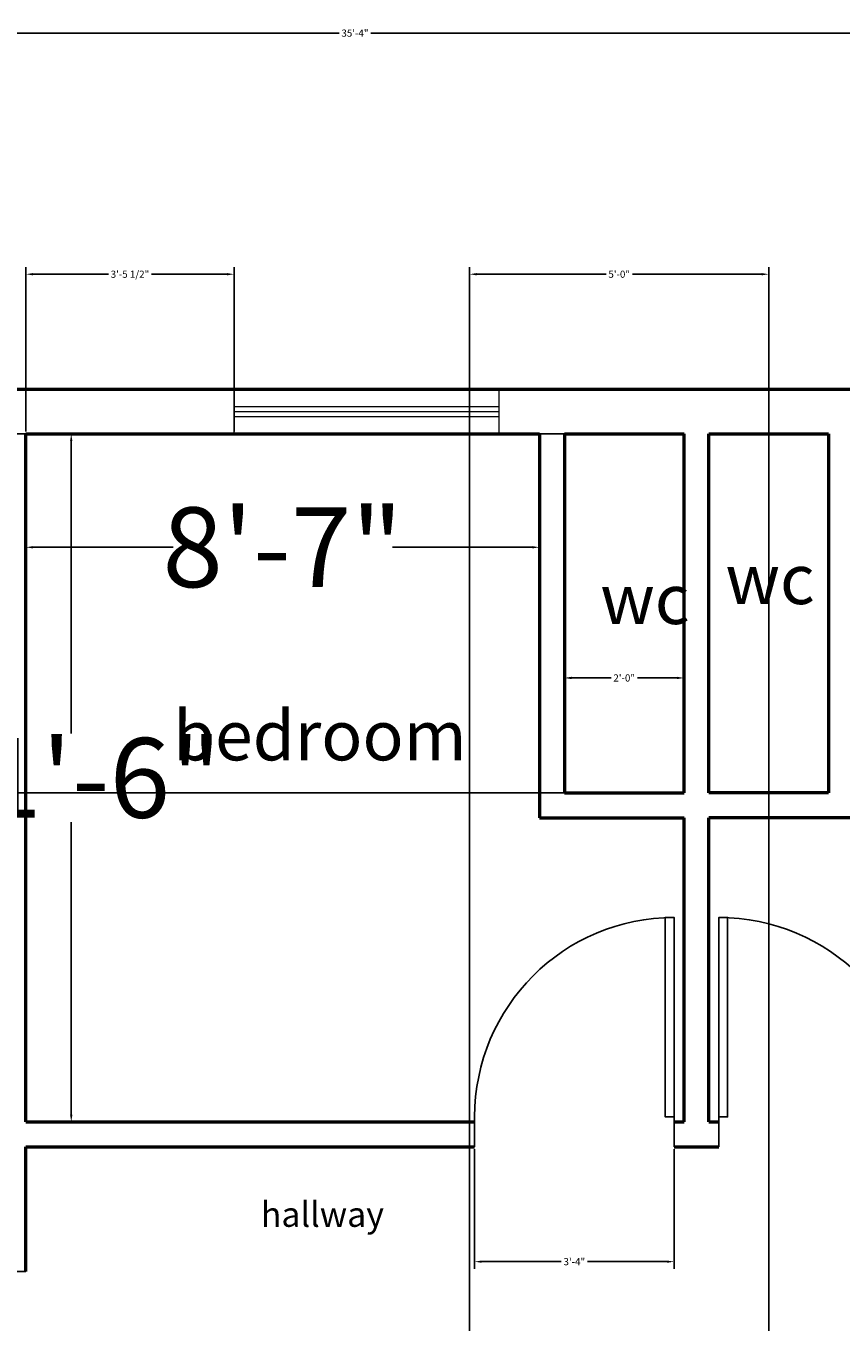
# Model space of a CAD drawing. Units: inches. Extents: x 325 to 804, y 366 to 834.
# Tile 5 of 6: x 496 to 660, y 574 to 834. Entities that reach past the tile are written whole.
import ezdxf

# ---------------------------------------------------------------- set-up
doc = ezdxf.new("R2010")
doc.units = ezdxf.units.IN
doc.header["$MEASUREMENT"] = 0
doc.layers.get('0').update_dxf_attribs({"color": 4})
for name, color, linetype, lineweight in [('A-ANNO-DIMS', 2, 'Continuous', 18), ('A-AREA-IDEN', 7, 'Continuous', 25), ('A-WALL', 7, 'Continuous', 50), ('door', 10, 'Continuous', 25), ('window', 3, 'Continuous', 18)]:
    doc.layers.add(name, color=color, linetype=linetype, lineweight=lineweight)
doc.styles.get("Standard").update_dxf_attribs({"font": 'arial.ttf'})
doc.dimstyles.get("Standard").update_dxf_attribs({"dimscale": 8, "dimtxt": 0.18, "dimasz": 0.18, "dimexe": 0.18, "dimexo": 0.0625, "dimgap": 0.09, "dimtad": 0, "dimtih": 1, "dimtoh": 1, "dimdec": 0, "dimzin": 0, "dimdsep": 46, "dimlunit": 3, "dimtxsty": 'Standard', "dimcen": 0.09, "dimadec": 0, "dimazin": 0, "dimtfac": 1, "dimtdec": 0, "dimtofl": 0, "dimtmove": 0, "dimatfit": 3, "dimfxl": 1, "dimtolj": 1, "dimtzin": 0, "dimarcsym": 0})

# ---------------------------------------------------------------- blocks, each defined once
blk = doc.blocks.new('*U2')
for p, q in [((0, 0), (0, -6)), ((-40, 0), (-40, -6))]:
    blk.add_line(p, q)
blk.add_lwpolyline([(0, 0), (0, 40), (-1.75, 40), (-1.75, 0)], close=True)
blk.add_arc((0, 0), 40, 90, 180)
blk = doc.blocks.new('*U3')
for p, q in [((0, 0), (0, -6)), ((40, 0), (40, -6))]:
    blk.add_line(p, q)
blk.add_lwpolyline([(0, 0), (0, 40), (1.75, 40), (1.75, 0)], close=True)
blk.add_arc((0, 0), 40, 0, 90)
blk = doc.blocks.new('*D11')
at = {"layer": 'A-ANNO-DIMS', "color": 0, "lineweight": -2, "transparency": 16777216}
for p, q in [((496.47, 752.04), (496.47, 728.37)), ((599.47, 752.04), (599.47, 728.37)), ((497.91, 729.81), (525.98, 729.81)), ((598.03, 729.81), (569.97, 729.81))]:
    blk.add_line(p, q, dxfattribs=at)
at = {"layer": 'A-ANNO-DIMS', "color": 0, "transparency": 16777216}
for points in [[(497.91, 730.05), (497.91, 729.57), (496.47, 729.81)], [(598.03, 730.05), (598.03, 729.57), (599.47, 729.81)]]:
    blk.add_solid(points, dxfattribs=at)
at = {"layer": 'Defpoints', "color": 0, "transparency": 16777216}
for p in [(496.47, 752.54), (599.47, 752.54), (599.47, 729.81)]:
    blk.add_point(p, dxfattribs=at)
at = {"layer": 'A-ANNO-DIMS', "color": 0, "transparency": 16777216, "insert": (547.97, 729.81), "char_height": 1.44, "attachment_point": 5}
blk.add_mtext('\\A1;{\\H11.11111x;8\'-7"}', dxfattribs=at)
blk = doc.blocks.new('*D12')
at = {"layer": 'A-ANNO-DIMS', "color": 0, "lineweight": -2, "transparency": 16777216}
for p, q in [((496.97, 752.54), (507, 752.54)), ((505.56, 751.1), (505.56, 692.43)), ((505.56, 615.98), (505.56, 674.65)), ((496.97, 614.54), (507, 614.54))]:
    blk.add_line(p, q, dxfattribs=at)
at = {"layer": 'A-ANNO-DIMS', "color": 0, "transparency": 16777216}
for points in [[(505.32, 751.1), (505.8, 751.1), (505.56, 752.54)], [(505.32, 615.98), (505.8, 615.98), (505.56, 614.54)]]:
    blk.add_solid(points, dxfattribs=at)
at = {"layer": 'Defpoints', "color": 0, "transparency": 16777216}
for p in [(496.47, 752.54), (505.56, 752.54), (496.47, 614.54)]:
    blk.add_point(p, dxfattribs=at)
at = {"layer": 'A-ANNO-DIMS', "color": 0, "transparency": 16777216, "insert": (505.56, 683.54), "char_height": 1.44, "attachment_point": 5}
blk.add_mtext('\\A1;{\\H11.11111x;11\'-6"}', dxfattribs=at)
blk = doc.blocks.new('*D25')
at = {"layer": 'A-ANNO-DIMS', "color": 0, "lineweight": -2, "transparency": 16777216}
for p, q in [((350.47, 762.04), (350.47, 834.4)), ((351.91, 832.96), (559.28, 832.96)), ((773.03, 832.96), (565.67, 832.96)), ((774.47, 762.04), (774.47, 834.4))]:
    blk.add_line(p, q, dxfattribs=at)
at = {"layer": 'A-ANNO-DIMS', "color": 0, "transparency": 16777216}
for points in [[(351.91, 833.2), (351.91, 832.72), (350.47, 832.96)], [(773.03, 833.2), (773.03, 832.72), (774.47, 832.96)]]:
    blk.add_solid(points, dxfattribs=at)
at = {"layer": 'Defpoints', "color": 0, "transparency": 16777216}
for p in [(774.47, 832.96), (350.47, 761.54), (774.47, 761.54)]:
    blk.add_point(p, dxfattribs=at)
at = {"layer": 'A-ANNO-DIMS', "color": 0, "transparency": 16777216, "insert": (562.47, 832.96), "char_height": 1.44, "attachment_point": 5}
blk.add_mtext('\\A1;35\'-4"', dxfattribs=at)
blk = doc.blocks.new('WIN-53_14x9')
for p, q in [((0, 5.5), (53.14, 5.5)), ((0, 4.5), (53.14, 4.5)), ((0, 3.5), (53.14, 3.5))]:
    blk.add_line(p, q)
blk.add_lwpolyline([(0, 9), (53.14, 9), (53.14, 0), (0, 0)], close=True)
blk = doc.blocks.new('*D31')
at = {"layer": 'A-ANNO-DIMS', "color": 0, "lineweight": -2, "transparency": 16777216}
for p, q in [((496.47, 753.04), (496.47, 786.03)), ((538.21, 753.04), (538.21, 786.03)), ((497.91, 784.59), (513.03, 784.59)), ((536.77, 784.59), (521.65, 784.59))]:
    blk.add_line(p, q, dxfattribs=at)
at = {"layer": 'A-ANNO-DIMS', "color": 0, "transparency": 16777216}
for points in [[(497.91, 784.83), (497.91, 784.35), (496.47, 784.59)], [(536.77, 784.83), (536.77, 784.35), (538.21, 784.59)]]:
    blk.add_solid(points, dxfattribs=at)
at = {"layer": 'Defpoints', "color": 0, "transparency": 16777216}
for p in [(538.21, 784.59), (496.47, 752.54), (538.21, 752.54)]:
    blk.add_point(p, dxfattribs=at)
at = {"layer": 'A-ANNO-DIMS', "color": 0, "transparency": 16777216, "insert": (517.34, 784.59), "char_height": 1.44, "attachment_point": 5}
blk.add_mtext('\\A1;3\'-5 1/2"', dxfattribs=at)
blk = doc.blocks.new('*D36')
at = {"layer": 'A-ANNO-DIMS', "color": 0, "lineweight": -2, "transparency": 16777216}
for p, q in [((604.47, 681.04), (604.47, 705.03)), ((628.47, 681.04), (628.47, 705.03)), ((605.91, 703.59), (613.83, 703.59)), ((627.03, 703.59), (619.12, 703.59))]:
    blk.add_line(p, q, dxfattribs=at)
at = {"layer": 'A-ANNO-DIMS', "color": 0, "transparency": 16777216}
for points in [[(605.91, 703.83), (605.91, 703.35), (604.47, 703.59)], [(627.03, 703.83), (627.03, 703.35), (628.47, 703.59)]]:
    blk.add_solid(points, dxfattribs=at)
at = {"layer": 'Defpoints', "color": 0, "transparency": 16777216}
for p in [(628.47, 703.59), (604.47, 680.54), (628.47, 680.54)]:
    blk.add_point(p, dxfattribs=at)
at = {"layer": 'A-ANNO-DIMS', "color": 0, "transparency": 16777216, "insert": (616.47, 703.59), "char_height": 1.44, "attachment_point": 5}
blk.add_mtext('\\A1;2\'-0"', dxfattribs=at)
blk = doc.blocks.new('*D37')
at = {"layer": 'A-ANNO-DIMS', "color": 0, "lineweight": -2, "transparency": 16777216}
for p, q in [((627.97, 752.54), (325.98, 752.54)), ((327.42, 751.1), (327.42, 717.99)), ((327.42, 681.98), (327.42, 715.08)), ((627.97, 680.54), (325.98, 680.54))]:
    blk.add_line(p, q, dxfattribs=at)
at = {"layer": 'A-ANNO-DIMS', "color": 0, "transparency": 16777216}
for points in [[(327.18, 751.1), (327.66, 751.1), (327.42, 752.54)], [(327.18, 681.98), (327.66, 681.98), (327.42, 680.54)]]:
    blk.add_solid(points, dxfattribs=at)
at = {"layer": 'Defpoints', "color": 0, "transparency": 16777216}
for p in [(327.42, 752.54), (628.47, 752.54), (628.47, 680.54)]:
    blk.add_point(p, dxfattribs=at)
at = {"layer": 'A-ANNO-DIMS', "color": 0, "transparency": 16777216, "insert": (327.42, 716.54), "char_height": 1.44, "attachment_point": 5}
blk.add_mtext('\\A1;6\'-0"', dxfattribs=at)
blk = doc.blocks.new('*D38')
at = {"layer": 'A-ANNO-DIMS', "color": 0, "lineweight": -2, "transparency": 16777216}
for p, q in [((585.47, 401.04), (585.47, 786.03)), ((645.47, 401.04), (645.47, 786.03)), ((586.91, 784.59), (612.84, 784.59)), ((644.03, 784.59), (618.11, 784.59))]:
    blk.add_line(p, q, dxfattribs=at)
at = {"layer": 'A-ANNO-DIMS', "color": 0, "transparency": 16777216}
for points in [[(586.91, 784.83), (586.91, 784.35), (585.47, 784.59)], [(644.03, 784.83), (644.03, 784.35), (645.47, 784.59)]]:
    blk.add_solid(points, dxfattribs=at)
at = {"layer": 'Defpoints', "color": 0, "transparency": 16777216}
for p in [(645.47, 784.59), (585.47, 400.54), (645.47, 400.54)]:
    blk.add_point(p, dxfattribs=at)
at = {"layer": 'A-ANNO-DIMS', "color": 0, "transparency": 16777216, "insert": (615.47, 784.59), "char_height": 1.44, "attachment_point": 5}
blk.add_mtext('\\A1;5\'-0"', dxfattribs=at)
blk = doc.blocks.new('*D40')
at = {"layer": 'A-ANNO-DIMS', "color": 0, "lineweight": -2, "transparency": 16777216}
for p, q in [((586.47, 609.04), (586.47, 585.05)), ((626.47, 609.04), (626.47, 585.05)), ((587.91, 586.49), (603.84, 586.49)), ((625.03, 586.49), (609.11, 586.49))]:
    blk.add_line(p, q, dxfattribs=at)
at = {"layer": 'A-ANNO-DIMS', "color": 0, "transparency": 16777216}
for points in [[(587.91, 586.73), (587.91, 586.25), (586.47, 586.49)], [(625.03, 586.73), (625.03, 586.25), (626.47, 586.49)]]:
    blk.add_solid(points, dxfattribs=at)
at = {"layer": 'Defpoints', "color": 0, "transparency": 16777216}
for p in [(586.47, 609.54), (626.47, 609.54), (586.47, 586.49)]:
    blk.add_point(p, dxfattribs=at)
at = {"layer": 'A-ANNO-DIMS', "color": 0, "transparency": 16777216, "insert": (606.47, 586.49), "char_height": 1.44, "attachment_point": 5}
blk.add_mtext('\\A1;3\'-4"', dxfattribs=at)

msp = doc.modelspace()

# ---------------------------------------------------------------- linework, layer by layer
at = {"layer": 'A-WALL'}
for p, q in [((350.47, 761.54), (774.47, 761.54)), ((496.47, 752.54), (599.47, 752.54)), ((496.47, 614.54), (496.47, 752.54)), ((599.47, 752.54), (599.47, 675.54)), ((604.47, 752.54), (604.47, 680.54)), ((604.47, 752.54), (628.47, 752.54)), ((628.47, 680.54), (628.47, 752.54)), ((633.47, 752.54), (657.47, 752.54)), ((633.47, 680.54), (633.47, 752.54)), ((657.47, 752.54), (657.47, 680.54)), ((604.47, 680.54), (628.47, 680.54)), ((657.47, 680.54), (633.47, 680.54)), ((599.47, 675.54), (628.47, 675.54)), ((628.47, 614.54), (628.47, 675.54)), ((633.47, 614.54), (633.47, 675.54)), ((662.47, 675.54), (633.47, 675.54)), ((496.47, 614.54), (586.47, 614.54)), ((626.47, 614.54), (628.47, 614.54)), ((633.47, 614.54), (635.47, 614.54)), ((496.47, 609.54), (586.47, 609.54)), ((496.47, 584.54), (496.47, 609.54)), ((626.47, 609.54), (635.47, 609.54))]:
    msp.add_line(p, q, dxfattribs=at)
at = {"layer": 'door'}
for p, q in [((626.47, 614.54), (626.47, 609.54)), ((635.47, 614.54), (635.47, 609.54))]:
    msp.add_line(p, q, dxfattribs=at)

# ---------------------------------------------------------------- block references
msp.add_blockref('*U2', (626.47, 615.54), dxfattribs=at)
at = {"layer": 'door', "xscale": -1}
msp.add_blockref('*U2', (635.47, 615.54), dxfattribs=at)
at = {"layer": 'door', "rotation": 90}
msp.add_blockref('*U3', (490.47, 544.54), dxfattribs=at)
at = {"layer": 'window'}
msp.add_blockref('WIN-53_14x9', (538.21, 752.54), dxfattribs=at)

# ---------------------------------------------------------------- texts
at = {"layer": 'A-AREA-IDEN', "attachment_point": 1}
for s, width, insert, char_height in [('wc', 25.6907, (636.78, 728.41), 10), ('wc', 25.6907, (611.67, 724.41), 10), ('bedroom', 79.8504, (525.97, 697.06), 10), ('hallway', 75.9333, (543.57, 598.47), 5)]:
    msp.add_mtext_dynamic_manual_height_columns(s, width=width, gutter_width=1, heights=[0], dxfattribs=dict(at, insert=insert, char_height=char_height))

# ---------------------------------------------------------------- dimensions: what is measured, and where the dimension line sits
at = {"layer": 'A-ANNO-DIMS'}
for base, p1, p2, override, picture, middle in [((774.47, 832.96), (350.47, 761.54), (774.47, 761.54), {"dimclrd": 0, "dimclre": 0, "dimclrt": 0}, '*D25', (562.47, 832.96)), ((538.21, 784.59), (496.47, 752.54), (538.21, 752.54), {"dimdec": 1, "dimlfac": 1, "dimrnd": 0, "dimzin": 1, "dimdsep": 46, "dimlunit": 4, "dimfrac": 2}, '*D31', (517.34, 784.59)), ((645.47, 784.59), (585.47, 400.54), (645.47, 400.54), {"dimdec": 1, "dimlfac": 1, "dimrnd": 0, "dimzin": 1, "dimdsep": 46, "dimlunit": 4, "dimfrac": 2}, '*D38', (615.47, 784.59)), ((628.47, 703.59), (604.47, 680.54), (628.47, 680.54), {"dimdec": 1, "dimlfac": 1, "dimrnd": 0, "dimzin": 1, "dimdsep": 46, "dimlunit": 4, "dimfrac": 2}, '*D36', (616.47, 703.59))]:
    dim = msp.add_linear_dim(base=base, p1=p1, p2=p2, dimstyle='Standard', override=override, dxfattribs=at)
    dim.commit()
    dim.dimension.update_dxf_attribs({"geometry": picture, "text_midpoint": middle})
for base, p1, p2, angle, picture, middle in [((327.42, 752.54), (628.47, 680.54), (628.47, 752.54), 90, '*D37', (327.42, 716.54)), ((586.47, 586.49), (626.47, 609.54), (586.47, 609.54), 180, '*D40', (606.47, 586.49))]:
    dim = msp.add_linear_dim(base=base, p1=p1, p2=p2, angle=angle, dimstyle='Standard', override={"dimdec": 1, "dimlfac": 1, "dimrnd": 0, "dimzin": 1, "dimdsep": 46, "dimlunit": 4, "dimfrac": 2}, dxfattribs=at)
    dim.commit()
    dim.dimension.update_dxf_attribs({"geometry": picture, "text_midpoint": middle})
dim = msp.add_linear_dim(base=(505.56, 752.54), p1=(496.47, 614.54), p2=(496.47, 752.54), angle=90, text='{\\H11.11111x;<>}', dimstyle='Standard', override={"dimclrd": 0, "dimclre": 0, "dimclrt": 0}, dxfattribs=at)
dim.commit()
dim.dimension.update_dxf_attribs({"geometry": '*D12', "text_midpoint": (505.56, 683.54)})
dim = msp.add_linear_dim(base=(599.47, 729.81), p1=(496.47, 752.54), p2=(599.47, 752.54), text='{\\H11.11111x;<>}', dimstyle='Standard', override={"dimclrd": 0, "dimclre": 0, "dimclrt": 0}, dxfattribs=at)
dim.commit()
dim.dimension.update_dxf_attribs({"geometry": '*D11', "text_midpoint": (547.97, 729.81)})

doc.saveas('drawing.dxf')
